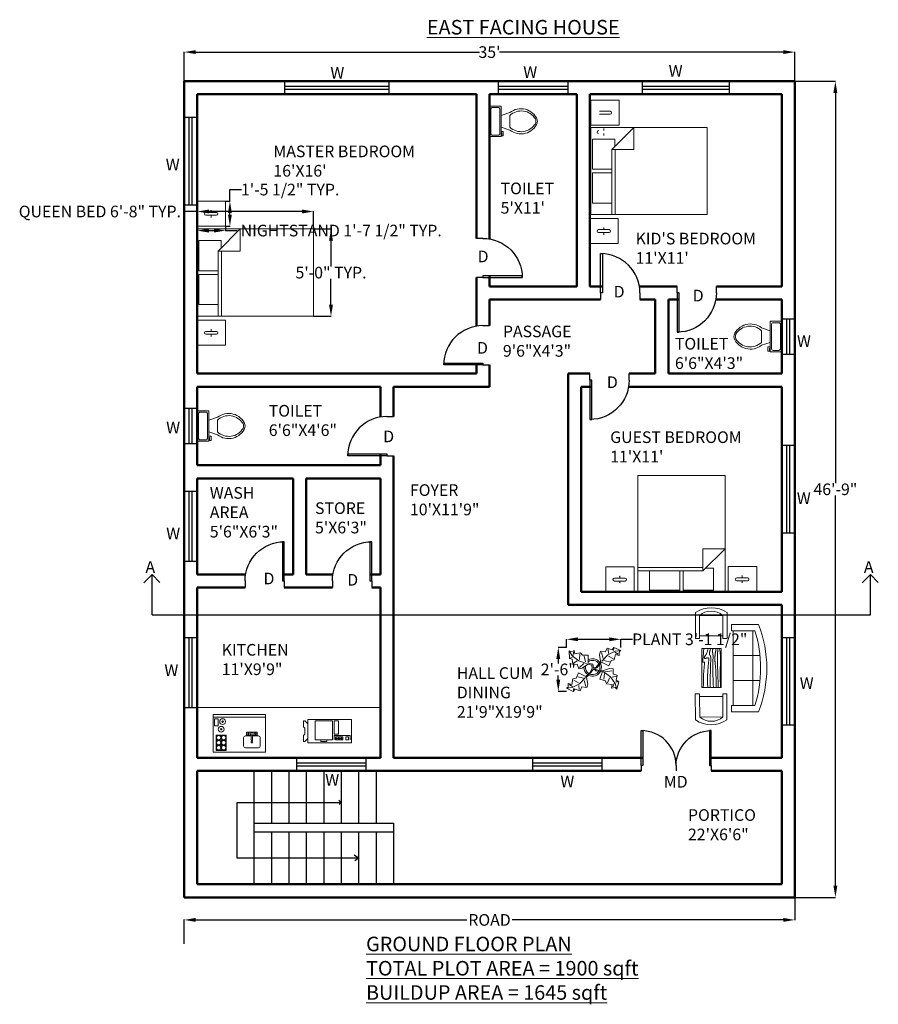
# Model space of a CAD drawing. Units: inches. Extents: x 179 to 2009, y 628 to 2084.
# Tile 1 of 5: x 179 to 769, y 628 to 1305. Entities that reach past the tile are written whole.
import ezdxf

# ---------------------------------------------------------------- set-up
doc = ezdxf.new("R2010")
doc.units = ezdxf.units.IN
doc.header["$MEASUREMENT"] = 0
for name, color, linetype, lineweight in [('A-ANNO-DIMS', 2, 'Continuous', 18), ('A-ANNO-SYMB', 5, 'Continuous', 25), ('A-ANNO-TEXT', 7, 'Continuous', 18), ('A-DOOR', 3, 'Continuous', 25), ('A-FLOR-STRS', 6, 'Continuous', 25), ('A-FURN', 4, 'Continuous', 18), ('A-GLAZ', 2, 'Continuous', 25), ('A-WALL', 1, 'Continuous', 50)]:
    doc.layers.add(name, color=color, linetype=linetype, lineweight=lineweight)
doc.styles.get("Standard").update_dxf_attribs({"font": 'arial.ttf'})
doc.dimstyles.get("Standard").update_dxf_attribs({"dimtxt": 8, "dimasz": 8, "dimexe": 0.18, "dimexo": 0.0625, "dimgap": 0.09, "dimtad": 0, "dimtih": 1, "dimtoh": 1, "dimdec": 0, "dimzin": 0, "dimdsep": 46, "dimlunit": 3, "dimtxsty": 'Standard', "dimcen": 0.09, "dimadec": 0, "dimazin": 0, "dimtfac": 1, "dimtdec": 0, "dimtofl": 0, "dimtmove": 0, "dimatfit": 3, "dimfxl": 1, "dimtolj": 1, "dimtzin": 0, "dimarcsym": 0})

# ---------------------------------------------------------------- blocks, each defined once
blk = doc.blocks.new('*U4')
for p, q in [((0, 0), (0, -6)), ((36, 0), (36, -6))]:
    blk.add_line(p, q)
blk.add_lwpolyline([(0, 0), (0, 36), (1.75, 36), (1.75, 0)], close=True)
blk.add_arc((0, 0), 36, 0, 90)
blk = doc.blocks.new('*U1')
for p, q in [((0, 0), (0, -6)), ((40, 0), (40, -6))]:
    blk.add_line(p, q)
blk.add_lwpolyline([(0, 0), (0, 40), (1.75, 40), (1.75, 0)], close=True)
blk.add_arc((0, 0), 40, 0, 90)
blk = doc.blocks.new('Bed - Queen')
for p, q in [((0, -80.00003), (0, 0)), ((0, 0), (59.99999, 0)), ((59.99999, 0), (59.99999, -80.00003)), ((7.99999, -1.2), (28.79998, -1.2)), ((7.99999, -14.4), (7.99999, -1.2)), ((28.79998, -1.2), (28.79998, -14.4)), ((31.19999, -1.2), (51.99999, -1.2)), ((31.19999, -14.4), (31.19999, -1.2)), ((51.99999, -1.2), (51.99999, -16.4)), ((0, -14.4), (44.8, -14.4)), ((44.8, -16.8), (0, -16.8)), ((59.99999, -29.6), (44.8, -14.4)), ((44.8, -14.4), (44.8, -29.6)), ((51.99999, -16.4), (46.79936, -16.4)), ((44.8, -29.6), (59.99999, -29.6)), ((59.99999, -80.00003), (0, -80.00003))]:
    blk.add_line(p, q)
blk = doc.blocks.new('*U3')
for p, q in [((9.5, -6), (9.5, -2)), ((-10, -8.5), (-8, -8.5)), ((-10, -9.5), (-10, -8.5)), ((-7, -9.5), (-10, -9.5)), ((-8, -8.5), (-8, -8)), ((-7, -8), (-7, -9.5)), ((-4, -8), (-6, -14)), ((4, -8), (6, -14)), ((4, -14), (-4, -14))]:
    blk.add_line(p, q)
blk.add_lwpolyline([(10.5, -8), (10.5, 0), (-10.5, 0), (-10.5, -8)], close=True)
for points in [[(-9.5, -2), (-9.5, -6)], [(8.5, -1), (-8.5, -1)], [(-8.5, -7), (8.5, -7)]]:
    blk.add_lwpolyline(points)
for centre, radius, start, end in [((-8.62, -1.88), 0.884, 81.8699, 188.1301), ((-8.62, -6.12), 0.884, 171.8699, 278.1301), ((8.62, -1.88), 0.884, 351.8699, 98.1301), ((8.62, -6.12), 0.884, 261.8699, 8.1301), ((3.52, -21.58), 12.17, 141.46911, 247.97143), ((4.2, -21.82), 11.33, 136.36773, 238.94682), ((-3.52, -21.58), 12.17, 292.02843, 38.53071), ((-4.2, -21.82), 11.33, 301.05301, 43.63209), ((0, -27.88), 4, 245.73182, 294.26817), ((0, -29), 4, 254.86053, 285.13947)]:
    blk.add_arc(centre, radius, start, end)
blk = doc.blocks.new('Wet Bar')
for p, q in [((0, 0), (36, 0)), ((0, -26), (0, 0)), ((36, 0), (36, -26)), ((0, -2), (36, -2)), ((3.5, -3), (1, -3)), ((1, -3), (1, -8)), ((3.5, -8), (3.5, -3)), ((1, -8), (3.5, -8)), ((2, -14.25), (9, -14.25)), ((2, -24.75), (2, -14.25)), ((2, -17.75), (9, -17.75)), ((5.5, -14.25), (5.5, -24.75)), ((9, -14.25), (9, -24.75)), ((26.2, -17.55), (26.2, -14.1284)), ((27.1001, -17.55), (27.1001, -14.1284)), ((36, -26), (0, -26)), ((9, -21.25), (2, -21.25)), ((9, -24.75), (2, -24.75))]:
    blk.add_line(p, q)
for points in [[(26.2, -14.25), (22.95, -14.25), (22.95, -12.2), (26.75, -12.2)], [(26.7487, -12.2), (30.3501, -12.2), (30.3501, -14.25), (27.1001, -14.25)], [(20.95, -21.75), (20.95, -16.05)], [(22.15, -14.85), (26.2, -14.85)], [(27.1001, -14.85), (31.15, -14.85)], [(32.3501, -16.05), (32.3501, -21.75)], [(31.15, -22.95), (22.15, -22.95)]]:
    blk.add_lwpolyline(points)
for centre, radius in [((6.5, -5), 2), ((6.5, -5), 0.5), ((5.5, -10.25), 2), ((5.5, -10.25), 0.5), ((24.25, -13.25), 0.5), ((26.65, -13.35), 0.9), ((29, -13.25), 0.5), ((3.75, -16), 1.5), ((3.75, -19.5), 1.5), ((7.25, -16), 1.5), ((7.25, -19.5), 1.5), ((26.65, -19.05), 0.6), ((3.75, -23), 1.5), ((7.25, -23), 1.5)]:
    blk.add_circle(centre, radius)
for centre, radius, start, end in [((22.2251, -16.125), 1.2772, 93.36646, 176.6335), ((26.65, -17.55), 0.45, 180, 0), ((31.075, -16.125), 1.2772, 3.366461, 86.63354), ((22.2251, -21.675), 1.2772, 183.3665, 266.6335), ((31.075, -21.675), 1.2772, 273.3665, 356.6335)]:
    blk.add_arc(centre, radius, start, end)
blk = doc.blocks.new('Copy Machine')
for p, q in [((0, 0), (0, -16)), ((30, 0), (0, 0)), ((30, -16), (30, 0)), ((-3, -1), (-3, -5)), ((-2, -1), (-3, -1)), ((-3, -5), (-2, -6)), ((0, -3), (-2, -1)), ((-2, -10), (-2, -6)), ((5, -1), (5, -14)), ((17, -1), (5, -1)), ((17, -14), (17, -1)), ((18, -1), (18, -10)), ((21, -1), (18, -1)), ((21, -10), (21, -1)), ((-3, -11), (-2, -10)), ((-3, -15), (-3, -11)), ((0, -13), (-2, -15)), ((18, -10), (21, -10)), ((18, -14), (18, -11)), ((18, -11), (29, -11)), ((24, -12), (19, -12)), ((19, -12), (19, -14)), ((24, -13), (19, -13)), ((20, -12), (20, -14)), ((21, -14), (21, -12)), ((22, -12), (22, -14)), ((23, -14), (23, -12)), ((24, -14), (24, -12)), ((28, -12), (26, -12)), ((26, -12), (26, -14)), ((28, -14), (28, -12)), ((29, -11), (29, -14)), ((-2, -15), (-3, -15)), ((0, -16), (30, -16)), ((5, -14), (17, -14)), ((9, -14), (9, -15)), ((9, -15), (13, -15)), ((13, -15), (13, -14)), ((19, -14), (24, -14)), ((26, -14), (28, -14))]:
    blk.add_line(p, q)
blk = doc.blocks.new('Sofa - Roundback 7 ft.')
for p, q in [((-12.00002, -32.4421), (-12.00003, -6.5971)), ((11.99997, -32.4421), (11.99998, -6.5971)), ((-36.000027, -34), (-36.000027, -11.4696)), ((-35.999844, -13.3819), (35.9998, -13.3819)), ((35.99998, -34), (35.99998, -11.4696)), ((-36.000027, -32.4421), (35.99998, -32.4421))]:
    blk.add_line(p, q)
for points in [[(-36.000027, -34), (-42.000027, -34), (-42.000027, -8)], [(41.99998, -8), (41.99998, -34), (35.99998, -34)]]:
    blk.add_lwpolyline(points)
for centre, radius, start, end in [((0, -114.25), 114.25, 68.43141, 111.5686), ((-0.00001, -127.1968), 121.1968, 72.72033, 107.2797)]:
    blk.add_arc(centre, radius, start, end)
blk = doc.blocks.new('Table - Rectangular Woodgrain 60 x 30 in.')
for p, q in [((0, 0), (0, -30)), ((60, 0), (0, 0)), ((60, -30), (60, 0)), ((0, -30), (60, -30))]:
    blk.add_line(p, q)
for points in [[(0, -2.4), (4.8155, -2.418), (9.0302, -2.4688), (12.709, -2.5477), (15.9167, -2.65), (18.7181, -2.7711), (21.1781, -2.9063), (23.3616, -3.0508), (25.3333, -3.2), (27.1477, -3.3495), (28.8172, -3.4958), (30.3437, -3.636), (31.7291, -3.7667), (32.9756, -3.8849), (34.0849, -3.9875), (35.059, -4.0714), (35.9, -4.1334), (36.6114, -4.1711), (37.2041, -4.1854), (37.6906, -4.1779), (38.0833, -4.15), (38.3948, -4.1034), (38.6375, -4.0396), (38.8239, -3.9602), (38.9666, -3.8667), (39.0764, -3.7608), (39.1573, -3.6448), (39.2116, -3.521), (39.2416, -3.3917), (39.2498, -3.2593), (39.2385, -3.1261), (39.21, -2.9944), (39.1666, -2.8667), (39.111, -2.7447), (39.0468, -2.6281), (38.978, -2.5163), (38.9083, -2.4083), (38.8418, -2.3035), (38.7823, -2.201), (38.7337, -2.1001), (38.7, -2), (38.6844, -1.9003), (38.6875, -1.8021), (38.7094, -1.707), (38.75, -1.6167), (38.8094, -1.5326), (38.8875, -1.4563), (38.9844, -1.3893), (39.1, -1.3333), (39.2351, -1.2896), (39.3937, -1.2583), (39.5804, -1.2396), (39.8, -1.2333), (40.057, -1.2396), (40.3562, -1.2583), (40.7023, -1.2896), (41.1, -1.3333), (41.5547, -1.3895), (42.0755, -1.4573), (42.6721, -1.5361), (43.3542, -1.625), (44.1316, -1.7233), (45.014, -1.8302), (46.0114, -1.9449), (47.1333, -2.0667), (48.3862, -2.1947), (49.7625, -2.3281), (51.2513, -2.4663), (52.8416, -2.6083), (54.5226, -2.7535), (56.2833, -2.9011), (58.1127, -3.0501), (60, -3.2)], [(0, -9.2), (6.5759, -9.0858), (11.9385, -9.0365), (16.2527, -9.0418), (19.6833, -9.0917), (22.3952, -9.1759), (24.5531, -9.2844), (26.322, -9.4069), (27.8666, -9.5333), (29.3241, -9.6553), (30.7203, -9.7719), (32.0532, -9.8837), (33.3208, -9.9917), (34.5213, -10.0965), (35.6526, -10.199), (36.7128, -10.2999), (37.7, -10.4), (38.6129, -10.4996), (39.4531, -10.5969), (40.223, -10.6895), (40.925, -10.775), (41.5613, -10.8512), (42.1344, -10.9156), (42.6465, -10.966), (43.1, -11), (43.4976, -11.0158), (43.8437, -11.0136), (44.143, -10.9942), (44.4, -10.9583), (44.6195, -10.9069), (44.8062, -10.8406), (44.9648, -10.7603), (45.1, -10.6667), (45.2155, -10.5598), (45.3114, -10.4365), (45.3871, -10.2929), (45.4416, -10.125), (45.4743, -9.929), (45.4844, -9.7011), (45.4709, -9.4371), (45.4333, -9.1333), (45.3716, -8.7883), (45.2896, -8.4104), (45.1919, -8.0107), (45.0833, -7.6), (44.9685, -7.1893), (44.8521, -6.7896), (44.7388, -6.4117), (44.6333, -6.0667), (44.54, -5.7628), (44.4614, -5.4979), (44.4001, -5.2675), (44.3583, -5.0667), (44.3384, -4.8909), (44.3427, -4.7354), (44.3736, -4.5956), (44.4333, -4.4667), (44.5236, -4.3453), (44.6427, -4.2333), (44.7884, -4.1339), (44.9583, -4.05), (45.1501, -3.9849), (45.3614, -3.9417), (45.59, -3.9234), (45.8333, -3.9333), (46.0915, -3.9749), (46.3734, -4.0531), (46.6906, -4.1736), (47.0542, -4.3417), (47.4756, -4.5629), (47.9661, -4.8427), (48.5372, -5.1866), (49.2, -5.6), (49.9676, -6.0844), (50.8594, -6.625), (51.8965, -7.2031), (53.1, -7.8), (54.491, -8.3969), (56.0906, -8.975), (57.9199, -9.5156), (60, -10)], [(0, -12.8), (5.1847, -12.9322), (9.6213, -13.0323), (13.3963, -13.1059), (16.5958, -13.1583), (19.3063, -13.1952), (21.614, -13.2219), (23.6054, -13.2439), (25.3666, -13.2667), (26.9728, -13.2947), (28.4531, -13.3281), (29.8256, -13.3663), (31.1083, -13.4083), (32.3191, -13.4535), (33.476, -13.501), (34.597, -13.5501), (35.7, -13.6), (36.7984, -13.6497), (37.8875, -13.6979), (38.9578, -13.743), (40, -13.7833), (41.0047, -13.8174), (41.9625, -13.8438), (42.864, -13.8607), (43.7, -13.8667), (44.4631, -13.8604), (45.1552, -13.8417), (45.7801, -13.8104), (46.3416, -13.7667), (46.8439, -13.7104), (47.2906, -13.6417), (47.6858, -13.5604), (48.0333, -13.4667), (48.3375, -13.3608), (48.6042, -13.2448), (48.8396, -13.121), (49.05, -12.9917), (49.2417, -12.8593), (49.4208, -12.7261), (49.5937, -12.5944), (49.7667, -12.4667), (49.9452, -12.3451), (50.1323, -12.2313), (50.3303, -12.1268), (50.5416, -12.0333), (50.7686, -11.9524), (51.0135, -11.8854), (51.2788, -11.8341), (51.5666, -11.8), (51.8785, -11.7843), (52.2116, -11.7865), (52.562, -11.8059), (52.926, -11.8417), (53.2998, -11.8931), (53.6795, -11.9594), (54.0614, -12.0397), (54.4416, -12.1333), (54.8223, -12.2401), (55.2293, -12.3625), (55.6942, -12.5037), (56.2489, -12.6667), (56.9251, -12.8547), (57.7545, -13.0708), (58.7689, -13.3182), (60, -13.6)], [(0, -18), (5.124, -17.7273), (9.6609, -17.5057), (13.6705, -17.3303), (17.2125, -17.1958), (20.3467, -17.0973), (23.1328, -17.0297), (25.6307, -16.9878), (27.9, -16.9667), (29.9928, -16.9617), (31.9302, -16.9703), (33.7254, -16.9907), (35.3917, -17.0208), (36.9423, -17.0588), (38.3906, -17.1026), (39.7499, -17.1503), (41.0333, -17.2), (42.2519, -17.2496), (43.4073, -17.2969), (44.4986, -17.3395), (45.525, -17.375), (46.4858, -17.4012), (47.3802, -17.4156), (48.2074, -17.416), (48.9667, -17.4), (49.6583, -17.3662), (50.2872, -17.3167), (50.8595, -17.2547), (51.3812, -17.1833), (51.8584, -17.1057), (52.2971, -17.025), (52.7034, -16.9443), (53.0833, -16.8667), (53.443, -16.7951), (53.789, -16.7313), (54.128, -16.6768), (54.4666, -16.6334), (54.8115, -16.6024), (55.1693, -16.5854), (55.5465, -16.5841), (55.95, -16.6), (56.3828, -16.6337), (56.8346, -16.6823), (57.2915, -16.7418), (57.7396, -16.8084), (58.165, -16.878), (58.5539, -16.9469), (58.8924, -17.0111), (59.1666, -17.0667), (59.3679, -17.1107), (59.5078, -17.1438), (59.6032, -17.1675), (59.6708, -17.1833), (59.7275, -17.193), (59.7901, -17.1979), (59.8753, -17.1998), (60, -17.2)], [(0, -22.4), (8.0098, -22.2501), (14.4094, -22.1011), (19.4168, -21.9535), (23.25, -21.8083), (26.1269, -21.6663), (28.2656, -21.5281), (29.884, -21.3947), (31.2, -21.2667), (32.3967, -21.1448), (33.5172, -21.0292), (34.5697, -20.9198), (35.5625, -20.8167), (36.5037, -20.7198), (37.4015, -20.6292), (38.2642, -20.5448), (39.1, -20.4667), (39.9164, -20.3951), (40.7187, -20.3313), (41.5117, -20.2768), (42.3, -20.2333), (43.0883, -20.2024), (43.8812, -20.1854), (44.6836, -20.1841), (45.5, -20.2), (46.3328, -20.234), (47.1747, -20.2844), (48.0163, -20.3488), (48.8479, -20.425), (49.66, -20.5106), (50.4429, -20.6031), (51.1872, -20.7004), (51.8833, -20.8), (52.5246, -20.8999), (53.1166, -20.9995), (53.6681, -21.0983), (54.1875, -21.1958), (54.6834, -21.2919), (55.1646, -21.3859), (55.6394, -21.4777), (56.1167, -21.5667), (56.6028, -21.6515), (57.0961, -21.7266), (57.5929, -21.7852), (58.0896, -21.8208), (58.5823, -21.8268), (59.0674, -21.7964), (59.5412, -21.723), (60, -21.6)], [(0, -25.2), (8.6355, -25.0504), (15.7026, -24.9031), (21.4049, -24.7606), (25.9458, -24.625), (29.529, -24.4988), (32.3578, -24.3844), (34.6359, -24.284), (36.5667, -24.2), (38.3213, -24.1341), (39.9417, -24.0854), (41.437, -24.0523), (42.8167, -24.0333), (44.0901, -24.0268), (45.2667, -24.0313), (46.3557, -24.0451), (47.3667, -24.0667), (48.309, -24.0947), (49.1928, -24.1287), (50.0284, -24.168), (50.826, -24.2125), (51.5959, -24.2617), (52.3483, -24.3151), (53.0935, -24.3725), (53.8417, -24.4334), (54.6009, -24.497), (55.3699, -24.561), (56.1454, -24.6226), (56.9239, -24.6792), (57.7021, -24.7279), (58.4764, -24.7662), (59.2435, -24.7911), (60, -24.8)], [(0, -28.8), (5.6867, -28.6681), (10.45, -28.5698), (14.407, -28.5012), (17.675, -28.4584), (20.3711, -28.4374), (22.6125, -28.4344), (24.5164, -28.4455), (26.2, -28.4667), (27.762, -28.4947), (29.2276, -28.5281), (30.6033, -28.5663), (31.8958, -28.6084), (33.1118, -28.6535), (34.2578, -28.7011), (35.3405, -28.7501), (36.3666, -28.8), (37.3443, -28.8497), (38.288, -28.8974), (39.2137, -28.9412), (40.1375, -28.9792), (41.0753, -29.0093), (42.0432, -29.0297), (43.0572, -29.0384), (44.1333, -29.0333), (45.2936, -29.0114), (46.5843, -28.9641), (48.0579, -28.8816), (49.7666, -28.7542), (51.7629, -28.5721), (54.0989, -28.3255), (56.8272, -28.0048), (60, -27.6)]]:
    blk.add_lwpolyline(points)
blk = doc.blocks.new('Plant - Rubber or Philodendron')
for p, q in [((13.3837, 12.301), (14.68, 13.9039)), ((14.68, 13.9039), (19.3848, 11.8146)), ((-16.2005, 11.4774), (-13.9899, 8.1064)), ((-16.2005, 11.4774), (-14.8639, 10.7964)), ((-16.0159, 6.3329), (-16.2005, 11.4774)), ((-15.3434, 6.5514), (-13.9984, 6.9884)), ((-14.8639, 10.7964), (-12.6195, 11.8975)), ((-13.9899, 8.1064), (-9.5434, 4.7185)), ((-13.3174, 8.325), (-13.0735, 11.0065)), ((-12.6195, 11.8975), (-12.1909, 9.4345)), ((-12.1909, 9.4345), (-8.3829, 10.3)), ((-8.8369, 9.409), (-9.0894, 5.6095)), ((-8.3829, 10.3), (-7.0549, 8.501)), ((-7.0549, 8.501), (-3.0284, 8.6941)), ((-4.8529, 4.012), (-5.7184, 7.82)), ((-3.0284, 8.6941), (-3.0709, 3.1041)), ((4.6914, 8.8812), (5.3859, 11.2828)), ((4.6914, 8.8812), (5.5014, 4.4831)), ((5.3859, 11.2828), (8.8871, 10.7908)), ((5.9878, 10.4842), (7.1971, 6.3869)), ((10.3916, 8.7942), (6.2847, 4.4028)), ((8.8871, 10.7908), (9.9809, 13.4933)), ((9.9809, 13.4933), (13.3837, 12.301)), ((15.3859, 11.3055), (10.3916, 8.7942)), ((10.5828, 12.6946), (10.8893, 9.7953)), ((14.2977, 6.1031), (10.9934, 7.9956)), ((14.5816, 13.2037), (14.3848, 11.8033)), ((15.7909, 9.1065), (14.8995, 5.3044)), ((15.2875, 10.6053), (17.5907, 9.2105)), ((19.3848, 11.8146), (15.3859, 11.3055)), ((18.1925, 8.4119), (15.7909, 9.1065)), ((19.3848, 11.8146), (18.1868, 10.9119)), ((18.1868, 10.9119), (18.1925, 8.4119)), ((-14.0069, 5.8704), (-16.0159, 6.3329)), ((-13.5868, 2.2894), (-14.0069, 5.8704)), ((-10.6784, 2.491), (-13.5868, 2.2894)), ((-13.1329, 3.1804), (-10.6614, 4.727)), ((-9.5858, -0.8715), (-10.6784, 2.491)), ((-9.5434, 4.7185), (-4.1917, 2.9888)), ((-9.1318, 0.0195), (-5.9793, 2.9025)), ((-7.1228, -0.443), (-3.5248, 2.2131)), ((-3.5248, 2.2131), (-3.3011, 2.4355)), ((-3.3011, 2.4355), (-0.5306, 1.7947)), ((-3.0709, 3.1041), (0.0797, 2.3163)), ((-0.5306, 1.7947), (-0.2255, -0.5527)), ((-0.5306, 1.7947), (-0.5306, 1.7947)), ((0.0797, 2.3163), (0.4866, -0.031)), ((0.4866, -0.031), (2.1141, 0.2298)), ((2.1141, 0.2298), (5.4346, 3.9146)), ((6.1032, 3.6844), (2.8262, -0.031)), ((5.4346, 3.9146), (5.5014, 4.4831)), ((11.1089, 1.1958), (6.1032, 3.6844)), ((7.7005, 4.8881), (11.5025, 3.9967)), ((12.7005, 4.8994), (11.1089, 1.1958)), ((14.8995, 5.3044), (12.7005, 4.8994)), ((-11.3237, -7.2629), (-9.7321, -3.5593)), ((-6.3237, -7.2516), (-10.1257, -6.3602)), ((-9.7321, -3.5593), (-4.7264, -6.0479)), ((-7.1228, -0.443), (-9.5858, -0.8715)), ((-2.019, -3.6148), (-4.7264, -6.0479)), ((-4.1246, -6.8466), (-4.0579, -6.2781)), ((-4.0579, -6.2781), (-0.9375, -3.1608)), ((-2.019, -3.6148), (-0.2255, -0.5527)), ((-0.9375, -3.1608), (0.5883, -0.8135)), ((0.5883, -0.8135), (2.2447, -2.0916)), ((2.8262, -0.031), (1.3003, -0.5527)), ((1.3003, -0.5527), (2.4193, -1.4655)), ((2.2447, -2.0916), (6.7108, -2.6626)), ((2.4193, -1.4655), (6.895, -2.1175)), ((4.943, -7.9659), (6.7108, -2.6626)), ((11.6605, -0.5413), (6.895, -2.1175)), ((12.3677, -6.1981), (7.219, -2.6772)), ((8.125, -4.0768), (7.7715, -7.9659)), ((8.3544, -2.7453), (13.1973, -2.1704)), ((11.6605, -0.5413), (14.1354, -0.8948)), ((15.5496, -10.7943), (12.3677, -6.1981)), ((16.2567, -5.8446), (13.4283, -6.5517)), ((14.1354, -0.8948), (14.1354, -4.4304)), ((14.1354, -4.4304), (16.9638, -5.1375)), ((16.9638, -5.1375), (16.2567, -8.673)), ((-18.008, -14.1781), (-16.8101, -13.2754)), ((-16.8157, -10.7754), (-14.4141, -11.4699)), ((-16.8101, -13.2754), (-16.8157, -10.7754)), ((-13.9107, -12.9688), (-16.2139, -11.574)), ((-14.4141, -11.4699), (-13.5228, -7.6679)), ((-14.0091, -13.669), (-9.0148, -11.1577)), ((-13.5228, -7.6679), (-11.3237, -7.2629)), ((-12.921, -8.4665), (-9.6166, -10.359)), ((-9.206, -15.0581), (-9.5126, -12.1588)), ((-9.0148, -11.1577), (-4.9047, -6.8122)), ((-7.5103, -13.1543), (-8.6042, -15.8568)), ((-4.0092, -13.6463), (-7.5103, -13.1543)), ((-4.611, -12.8477), (-5.8203, -8.7504)), ((-3.3146, -11.2447), (-4.1246, -6.8466)), ((-3.3146, -11.2447), (-4.0092, -13.6463)), ((8.8321, -9.0266), (4.943, -7.9659)), ((9.5392, -11.1479), (8.8321, -9.0266)), ((13.4283, -11.5015), (9.5392, -11.1479)), ((10.2463, -10.4408), (11.6605, -6.9053)), ((13.0748, -13.9763), (13.4283, -11.5015)), ((14.8425, -10.7943), (13.7819, -13.2692)), ((16.6103, -14.6834), (15.5496, -10.7943)), ((17.3174, -9.7337), (15.9032, -9.7337)), ((16.2567, -8.673), (18.0245, -9.7337)), ((18.0245, -9.7337), (16.6103, -14.6834)), ((-18.008, -14.1781), (-14.0091, -13.669)), ((-13.3032, -16.2674), (-18.008, -14.1781)), ((-12.0069, -14.6645), (-13.3032, -16.2674)), ((-13.2048, -15.5672), (-13.008, -14.1668)), ((-8.6042, -15.8568), (-12.0069, -14.6645)), ((15.5496, -13.6228), (13.0748, -13.9763)), ((16.6103, -14.6834), (15.5496, -13.6228))]:
    blk.add_line(p, q)
for centre, radius, start, end in [((0.0308, 0.1664), 6, 178.6147, 235.1169), ((0.0308, 0.1664), 5, 168.1647, 238.6725), ((0, 0), 6.1275, 34.37569, 120.1028), ((-0.0601, -0.2075), 5.2461, 33.82192, 124.9414), ((-0.2664, 0.1682), 5.2775, 338.4094, 20.03007), ((-0.098, 0.1364), 6.1288, 341.2017, 26.09184), ((-0.0234, 0.3825), 6.1492, 242.5812, 331.2714), ((-0.1102, 0.4886), 5.2883, 247.3711, 327.472)]:
    blk.add_arc(centre, radius, start, end)
blk = doc.blocks.new('*D14')
at = {"layer": 'A-ANNO-DIMS', "color": 0, "lineweight": -2, "transparency": 16777216}
for p, q in [((291.69, 1262.41), (291.69, 1282.56)), ((299.69, 1282.38), (494.81, 1282.38)), ((703.69, 1282.38), (508.56, 1282.38)), ((711.69, 1262.41), (711.69, 1282.56))]:
    blk.add_line(p, q, dxfattribs=at)
at = {"layer": 'A-ANNO-DIMS', "color": 0, "transparency": 16777216}
for points in [[(299.69, 1283.72), (299.69, 1281.05), (291.69, 1282.38)], [(703.69, 1283.72), (703.69, 1281.05), (711.69, 1282.38)]]:
    blk.add_solid(points, dxfattribs=at)
at = {"layer": 'Defpoints', "color": 0, "transparency": 16777216}
for p in [(711.69, 1282.38), (291.69, 1262.35), (711.69, 1262.35)]:
    blk.add_point(p, dxfattribs=at)
at = {"layer": 'A-ANNO-DIMS', "color": 0, "transparency": 16777216, "insert": (501.69, 1282.38), "char_height": 8, "attachment_point": 5}
blk.add_mtext("\\A1;35'", dxfattribs=at)
blk = doc.blocks.new('*D15')
at = {"layer": 'A-ANNO-DIMS', "color": 0, "lineweight": -2, "transparency": 16777216}
for p, q in [((711.75, 1262.35), (739.72, 1262.35)), ((739.54, 1254.35), (739.54, 986.02)), ((739.54, 709.35), (739.54, 977.68)), ((711.75, 701.35), (739.72, 701.35))]:
    blk.add_line(p, q, dxfattribs=at)
at = {"layer": 'A-ANNO-DIMS', "color": 0, "transparency": 16777216}
for points in [[(738.2, 1254.35), (740.87, 1254.35), (739.54, 1262.35)], [(738.2, 709.35), (740.87, 709.35), (739.54, 701.35)]]:
    blk.add_solid(points, dxfattribs=at)
at = {"layer": 'Defpoints', "color": 0, "transparency": 16777216}
for p in [(711.69, 1262.35), (711.69, 701.35), (739.54, 701.35)]:
    blk.add_point(p, dxfattribs=at)
at = {"layer": 'A-ANNO-DIMS', "color": 0, "transparency": 16777216, "insert": (739.54, 981.85), "char_height": 8, "attachment_point": 5}
blk.add_mtext('\\A1;46\'-9"', dxfattribs=at)
blk = doc.blocks.new('*D16')
at = {"layer": 'A-ANNO-DIMS', "color": 0, "lineweight": -2, "transparency": 16777216}
for p, q in [((711.69, 701.29), (711.69, 685.68)), ((291.69, 669.31), (291.69, 686.04)), ((299.69, 685.86), (486.19, 685.86)), ((703.69, 685.86), (517.18, 685.86))]:
    blk.add_line(p, q, dxfattribs=at)
at = {"layer": 'A-ANNO-DIMS', "color": 0, "transparency": 16777216}
for points in [[(299.69, 687.2), (299.69, 684.53), (291.69, 685.86)], [(703.69, 687.2), (703.69, 684.53), (711.69, 685.86)]]:
    blk.add_solid(points, dxfattribs=at)
at = {"layer": 'Defpoints', "color": 0, "transparency": 16777216}
for p in [(711.69, 701.35), (711.69, 685.86), (291.69, 669.25)]:
    blk.add_point(p, dxfattribs=at)
at = {"layer": 'A-ANNO-DIMS', "color": 0, "transparency": 16777216, "insert": (501.69, 685.86), "char_height": 8, "attachment_point": 5}
blk.add_mtext('\\A1;ROAD', dxfattribs=at)
blk = doc.blocks.new('ARMCHAIR')
for p, q in [((0, 0), (0, 17.87)), ((2.68, 1.83), (2.68, 15.94)), ((2.68, 15.94), (18.72, 15.94)), ((18.72, 15.94), (18.72, 1.83)), ((21.68, 0), (21.68, 17.87)), ((2.68, 0), (0, 0)), ((18.72, 1.83), (2.68, 1.83)), ((2.68, 1.83), (2.68, 0)), ((18.72, 1.83), (18.72, 0)), ((18.72, 0), (21.68, 0))]:
    blk.add_line(p, q)
for centre, radius, start, end in [((10.84, 2.23), 19.03, 55.27776, 124.72224), ((10.7, 6.48), 12.4, 49.71958, 130.28042)]:
    blk.add_arc(centre, radius, start, end)
blk = doc.blocks.new('NIGHTSTAND-2')
for p, q in [((5.95, 9.55), (13.25, 9.55)), ((5.95, 7.55), (13.25, 7.55)), ((9.6, 10.86), (9.43, 10.74)), ((9.6, 9.55), (9.6, 10.86)), ((9.6, 10.86), (9.78, 10.74)), ((9.6, 7.55), (9.6, 6.33)), ((9.6, 6.33), (9.37, 6.5)), ((9.6, 6.33), (9.83, 6.48))]:
    blk.add_line(p, q)
blk.add_lwpolyline([(0, 17.25), (19.57, 17.25), (19.57, 0), (0, 0)], close=True)
for centre, start, end in [((5.95, 8.55), 90, 270), ((13.25, 8.55), 270, 90)]:
    blk.add_arc(centre, 1, start, end)
blk = doc.blocks.new('*D43')
at = {"layer": 'A-ANNO-DIMS', "color": 0, "lineweight": -2, "transparency": 16777216}
for p, q in [((300.69, 1172.8), (292.69, 1172.8)), ((300.69, 1160.87), (300.69, 1172.98)), ((372.69, 1172.8), (308.69, 1172.8)), ((380.69, 1160.87), (380.69, 1172.98))]:
    blk.add_line(p, q, dxfattribs=at)
at = {"layer": 'A-ANNO-DIMS', "color": 0, "transparency": 16777216}
for points in [[(308.69, 1174.14), (308.69, 1171.47), (300.69, 1172.8)], [(372.69, 1174.14), (372.69, 1171.47), (380.69, 1172.8)]]:
    blk.add_solid(points, dxfattribs=at)
at = {"layer": 'Defpoints', "color": 0, "transparency": 16777216}
for p in [(300.69, 1172.8), (300.69, 1160.8), (380.69, 1160.8)]:
    blk.add_point(p, dxfattribs=at)
at = {"layer": 'A-ANNO-DIMS', "color": 0, "transparency": 16777216, "insert": (233.76, 1172.8), "char_height": 8, "attachment_point": 5}
blk.add_mtext('\\A1;QUEEN BED 6\'-8" TYP.', dxfattribs=at)
blk = doc.blocks.new('*D44')
at = {"layer": 'A-ANNO-DIMS', "color": 0, "lineweight": -2, "transparency": 16777216}
for p, q in [((380.75, 1160.8), (392.87, 1160.8)), ((392.69, 1152.8), (392.69, 1134.98)), ((392.69, 1108.8), (392.69, 1126.63)), ((380.75, 1100.8), (392.87, 1100.8))]:
    blk.add_line(p, q, dxfattribs=at)
at = {"layer": 'A-ANNO-DIMS', "color": 0, "transparency": 16777216}
for points in [[(391.35, 1152.8), (394.02, 1152.8), (392.69, 1160.8)], [(391.35, 1108.8), (394.02, 1108.8), (392.69, 1100.8)]]:
    blk.add_solid(points, dxfattribs=at)
at = {"layer": 'Defpoints', "color": 0, "transparency": 16777216}
for p in [(380.69, 1160.8), (392.69, 1160.8), (380.69, 1100.8)]:
    blk.add_point(p, dxfattribs=at)
at = {"layer": 'A-ANNO-DIMS', "color": 0, "transparency": 16777216, "insert": (392.69, 1130.8), "char_height": 8, "attachment_point": 5}
blk.add_mtext('\\A1;5\'-0" TYP.', dxfattribs=at)
blk = doc.blocks.new('*D49')
at = {"layer": 'A-ANNO-DIMS', "color": 0, "lineweight": -2, "transparency": 16777216}
for p, q in [((300.69, 1162.57), (300.69, 1159.52)), ((308.69, 1159.7), (312.25, 1159.7)), ((320.25, 1162.57), (320.25, 1159.52)), ((320.25, 1159.7), (328.25, 1159.7))]:
    blk.add_line(p, q, dxfattribs=at)
at = {"layer": 'A-ANNO-DIMS', "color": 0, "transparency": 16777216}
for points in [[(308.69, 1161.03), (308.69, 1158.36), (300.69, 1159.7)], [(312.25, 1161.03), (312.25, 1158.36), (320.25, 1159.7)]]:
    blk.add_solid(points, dxfattribs=at)
at = {"layer": 'Defpoints', "color": 0, "transparency": 16777216}
for p in [(300.69, 1162.63), (320.25, 1162.63), (320.25, 1159.7)]:
    blk.add_point(p, dxfattribs=at)
at = {"layer": 'A-ANNO-DIMS', "color": 0, "transparency": 16777216, "insert": (399.73, 1159.7), "char_height": 8, "attachment_point": 5}
blk.add_mtext('\\A1;NIGHTSTAND 1\'-7 1/2" TYP.', dxfattribs=at)
blk = doc.blocks.new('*D50')
at = {"layer": 'A-ANNO-DIMS', "color": 0, "lineweight": -2, "transparency": 16777216}
for p, q in [((323.19, 1179.88), (323.19, 1187.88)), ((323.19, 1187.88), (331.19, 1187.88)), ((320.31, 1179.88), (323.37, 1179.88)), ((323.19, 1170.63), (323.19, 1171.88)), ((320.31, 1162.63), (323.37, 1162.63))]:
    blk.add_line(p, q, dxfattribs=at)
at = {"layer": 'A-ANNO-DIMS', "color": 0, "transparency": 16777216}
for points in [[(321.85, 1171.88), (324.52, 1171.88), (323.19, 1179.88)], [(321.85, 1170.63), (324.52, 1170.63), (323.19, 1162.63)]]:
    blk.add_solid(points, dxfattribs=at)
at = {"layer": 'Defpoints', "color": 0, "transparency": 16777216}
for p in [(320.25, 1179.88), (323.19, 1179.88), (320.25, 1162.63)]:
    blk.add_point(p, dxfattribs=at)
at = {"layer": 'A-ANNO-DIMS', "color": 0, "transparency": 16777216, "insert": (364.6, 1187.88), "char_height": 8, "attachment_point": 5}
blk.add_mtext('\\A1;1\'-5 1/2" TYP.', dxfattribs=at)
blk = doc.blocks.new('*D61')
at = {"layer": 'A-ANNO-DIMS', "color": 0, "lineweight": -2, "transparency": 16777216}
for p, q in [((554.6, 873.19), (554.6, 878.92)), ((562.6, 878.74), (583.99, 878.74)), ((591.99, 873.19), (591.99, 878.92)), ((591.99, 878.74), (599.99, 878.74))]:
    blk.add_line(p, q, dxfattribs=at)
at = {"layer": 'A-ANNO-DIMS', "color": 0, "transparency": 16777216}
for points in [[(562.6, 880.07), (562.6, 877.41), (554.6, 878.74)], [(583.99, 880.07), (583.99, 877.41), (591.99, 878.74)]]:
    blk.add_solid(points, dxfattribs=at)
at = {"layer": 'Defpoints', "color": 0, "transparency": 16777216}
for p in [(554.6, 873.13), (591.99, 878.74), (591.99, 873.13)]:
    blk.add_point(p, dxfattribs=at)
at = {"layer": 'A-ANNO-DIMS', "color": 0, "transparency": 16777216, "insert": (639.4, 878.74), "char_height": 8, "attachment_point": 5}
blk.add_mtext('\\A1;PLANT 3\'-1 1/2"', dxfattribs=at)
blk = doc.blocks.new('*D62')
at = {"layer": 'A-ANNO-DIMS', "color": 0, "lineweight": -2, "transparency": 16777216}
for p, q in [((554.53, 873.13), (548.81, 873.13)), ((548.99, 865.13), (548.99, 862.22)), ((548.99, 850.96), (548.99, 853.87)), ((554.53, 842.96), (548.81, 842.96))]:
    blk.add_line(p, q, dxfattribs=at)
at = {"layer": 'A-ANNO-DIMS', "color": 0, "transparency": 16777216}
for points in [[(547.65, 865.13), (550.32, 865.13), (548.99, 873.13)], [(547.65, 850.96), (550.32, 850.96), (548.99, 842.96)]]:
    blk.add_solid(points, dxfattribs=at)
at = {"layer": 'Defpoints', "color": 0, "transparency": 16777216}
for p in [(548.99, 873.13), (554.6, 873.13), (554.6, 842.96)]:
    blk.add_point(p, dxfattribs=at)
at = {"layer": 'A-ANNO-DIMS', "color": 0, "transparency": 16777216, "insert": (548.99, 858.04), "char_height": 8, "attachment_point": 5}
blk.add_mtext('\\A1;2\'-6"', dxfattribs=at)

msp = doc.modelspace()

# ---------------------------------------------------------------- linework, layer by layer
at = {"layer": 'A-ANNO-SYMB'}
for p, q in [((269.72, 923.19), (263.96, 917.47)), ((269.72, 895.65), (269.72, 923.19)), ((269.72, 923.19), (275.04, 917.84)), ((763.74, 923.19), (757.98, 917.47)), ((763.74, 895.65), (763.74, 923.19)), ((763.74, 923.19), (769.06, 917.84)), ((269.72, 895.65), (763.74, 895.65))]:
    msp.add_line(p, q, dxfattribs=at)
at = {"layer": 'A-FLOR-STRS'}
for p, q in [((339.69, 788.35), (339.69, 710.35)), ((351.69, 788.35), (351.69, 752.35)), ((363.69, 788.35), (363.69, 752.35)), ((375.69, 788.35), (375.69, 752.35)), ((387.69, 788.35), (387.69, 752.35)), ((399.69, 788.35), (399.69, 752.35)), ((411.69, 788.35), (411.69, 752.35)), ((423.69, 788.35), (423.69, 752.35)), ((328.24, 728.35), (328.24, 766.55)), ((328.24, 766.55), (399.69, 766.55)), ((399.69, 766.55), (398.08, 767.97)), ((399.69, 766.55), (398.32, 765.27)), ((339.69, 752.35), (435.69, 752.35)), ((435.69, 752.35), (435.69, 710.35)), ((339.69, 746.35), (435.69, 746.35)), ((351.69, 746.35), (351.69, 710.35)), ((363.69, 746.35), (363.69, 710.35)), ((375.69, 746.35), (375.69, 710.35)), ((387.69, 746.35), (387.69, 710.35)), ((399.69, 746.35), (399.69, 710.35)), ((411.69, 746.35), (411.69, 710.35)), ((423.69, 746.35), (423.69, 710.35)), ((411.69, 728.35), (328.24, 728.35)), ((411.69, 728.35), (408.72, 730.27)), ((411.69, 728.35), (409.16, 726.46))]:
    msp.add_line(p, q, dxfattribs=at)
at = {"layer": 'A-FURN'}
for p, q in [((577.36, 1241.71), (584.66, 1241.71)), ((577.36, 1239.71), (584.66, 1239.71)), ((580.29, 1225.2), (580.05, 1225.36)), ((580.29, 1229.73), (580.11, 1229.6)), ((580.29, 1228.42), (580.29, 1229.73)), ((580.29, 1229.73), (580.47, 1229.61)), ((580.29, 1226.42), (580.29, 1225.2)), ((580.29, 1225.2), (580.52, 1225.34)), ((300.69, 831.85), (426.69, 831.85))]:
    msp.add_line(p, q, dxfattribs=at)
msp.add_lwpolyline([(571.41, 1249.41), (590.97, 1249.41), (590.97, 1232.16), (571.41, 1232.16)], close=True, dxfattribs=at)
for centre, start, end in [((584.66, 1240.71), 270, 90), ((576.64, 1227.42), 90, 270)]:
    msp.add_arc(centre, 1, start, end, dxfattribs=at)
at = {"layer": 'A-GLAZ'}
for p, q in [((360.69, 1258.85), (432.69, 1258.85)), ((360.69, 1256.85), (432.69, 1256.85)), ((507.69, 1258.85), (555.69, 1258.85)), ((507.69, 1256.85), (555.69, 1256.85)), ((606.69, 1258.85), (666.69, 1258.85)), ((606.69, 1256.85), (666.69, 1256.85)), ((295.19, 1177.46), (295.19, 1237.46)), ((297.19, 1177.46), (297.19, 1237.46)), ((706.19, 1074.85), (706.19, 1098.85)), ((708.19, 1074.85), (708.19, 1098.85)), ((295.19, 1013.35), (295.19, 1037.35)), ((297.19, 1013.35), (297.19, 1037.35)), ((706.19, 951.85), (706.19, 1011.85)), ((708.19, 951.85), (708.19, 1011.85)), ((295.19, 932.35), (295.19, 980.35)), ((297.19, 932.35), (297.19, 980.35)), ((295.19, 831.85), (295.19, 879.85)), ((297.19, 831.85), (297.19, 879.85)), ((706.19, 819.85), (706.19, 879.85)), ((708.19, 819.85), (708.19, 879.85)), ((368.86, 793.85), (416.86, 793.85)), ((531.27, 793.85), (579.27, 793.85)), ((368.86, 791.85), (416.86, 791.85)), ((531.27, 791.85), (579.27, 791.85))]:
    msp.add_line(p, q, dxfattribs=at)
for points in [[(360.69, 1253.35), (432.69, 1253.35), (432.69, 1262.35), (360.69, 1262.35)], [(507.69, 1253.35), (555.69, 1253.35), (555.69, 1262.35), (507.69, 1262.35)], [(606.69, 1253.35), (666.69, 1253.35), (666.69, 1262.35), (606.69, 1262.35)], [(300.69, 1177.46), (300.69, 1237.46), (291.69, 1237.46), (291.69, 1177.46)], [(711.69, 1074.85), (711.69, 1098.85), (702.69, 1098.85), (702.69, 1074.85)], [(300.69, 1013.35), (300.69, 1037.35), (291.69, 1037.35), (291.69, 1013.35)], [(711.69, 951.85), (711.69, 1011.85), (702.69, 1011.85), (702.69, 951.85)], [(300.69, 932.35), (300.69, 980.35), (291.69, 980.35), (291.69, 932.35)], [(300.69, 831.85), (300.69, 879.85), (291.69, 879.85), (291.69, 831.85)], [(711.69, 819.85), (711.69, 879.85), (702.69, 879.85), (702.69, 819.85)], [(368.86, 788.35), (416.86, 788.35), (416.86, 797.35), (368.86, 797.35)], [(531.27, 788.35), (579.27, 788.35), (579.27, 797.35), (531.27, 797.35)]]:
    msp.add_lwpolyline(points, close=True, dxfattribs=at)
at = {"layer": 'A-WALL'}
for p, q in [((291.69, 1262.35), (711.69, 1262.35)), ((291.69, 1262.35), (291.69, 701.35)), ((711.69, 1262.35), (711.69, 701.35)), ((300.69, 1253.35), (492.69, 1253.35)), ((300.69, 1253.35), (300.69, 1061.35)), ((492.69, 1253.35), (492.69, 1154.35)), ((501.69, 1253.35), (501.69, 1153.97)), ((501.69, 1253.35), (561.69, 1253.35)), ((561.69, 1253.35), (561.69, 1121.35)), ((570.69, 1253.35), (570.69, 1121.35)), ((570.69, 1253.35), (702.69, 1253.35)), ((702.69, 1253.35), (702.69, 1121.35)), ((492.69, 1127.35), (492.69, 1093.97)), ((501.69, 1128.66), (501.69, 1121.35)), ((501.69, 1121.35), (561.69, 1121.35)), ((570.69, 1121.35), (579.45, 1121.35)), ((604.75, 1121.35), (630.69, 1121.35)), ((657.69, 1121.35), (702.69, 1121.35)), ((501.69, 1112.35), (578.13, 1112.35)), ((501.69, 1112.35), (501.69, 1094.35)), ((605.13, 1112.35), (615.69, 1112.35)), ((615.69, 1112.35), (615.69, 1061.35)), ((624.69, 1112.35), (624.69, 1061.35)), ((624.69, 1112.35), (632, 1112.35)), ((657.31, 1112.35), (702.69, 1112.35)), ((702.69, 1112.35), (702.69, 1061.35)), ((492.69, 1068.66), (492.69, 1061.35)), ((501.69, 1067.35), (501.69, 1052.35)), ((300.69, 1061.35), (492.69, 1061.35)), ((555.69, 1061.35), (555.69, 902.35)), ((555.69, 1061.35), (570.69, 1061.35)), ((597.69, 1061.35), (615.69, 1061.35)), ((624.69, 1061.35), (702.69, 1061.35)), ((300.69, 1052.35), (426.69, 1052.35)), ((300.69, 1052.35), (300.69, 998.35)), ((426.69, 1052.35), (426.69, 1031.52)), ((435.69, 1052.35), (435.69, 1031.9)), ((435.69, 1052.35), (501.69, 1052.35)), ((492.69, 1052.35), (501.69, 1052.35)), ((564.69, 1052.35), (564.69, 911.35)), ((564.69, 1052.35), (572, 1052.35)), ((597.31, 1052.35), (702.69, 1052.35)), ((702.69, 1052.35), (702.69, 911.35)), ((426.69, 1006.21), (426.69, 998.35)), ((435.69, 1004.9), (435.69, 797.35)), ((300.69, 998.35), (426.69, 998.35)), ((300.69, 989.35), (366.69, 989.35)), ((300.69, 989.35), (300.69, 923.35)), ((366.69, 989.35), (366.69, 923.35)), ((375.69, 989.35), (375.69, 923.35)), ((375.69, 989.35), (426.69, 989.35)), ((426.69, 989.35), (426.69, 923.35)), ((300.69, 923.35), (333.98, 923.35)), ((359.29, 923.35), (366.69, 923.35)), ((375.69, 923.35), (394.06, 923.35)), ((419.37, 923.35), (426.69, 923.35)), ((300.69, 914.35), (333.6, 914.35)), ((300.69, 914.35), (300.69, 797.35)), ((360.6, 914.35), (393.69, 914.35)), ((420.69, 914.35), (426.69, 914.35)), ((426.69, 914.35), (426.69, 797.35)), ((564.69, 911.35), (702.69, 911.35)), ((555.69, 902.35), (702.69, 902.35)), ((702.69, 902.35), (702.69, 797.35)), ((300.69, 797.35), (426.69, 797.35)), ((435.69, 797.35), (607.08, 797.35)), ((652.98, 797.35), (702.69, 797.35)), ((300.69, 788.35), (606.03, 788.35)), ((300.69, 788.35), (300.69, 710.35)), ((654.03, 788.35), (702.69, 788.35)), ((702.69, 788.35), (702.69, 710.35)), ((300.69, 710.35), (702.69, 710.35)), ((291.69, 701.35), (711.69, 701.35))]:
    msp.add_line(p, q, dxfattribs=at)

# ---------------------------------------------------------------- block references
at = {"layer": 'A-DOOR', "yscale": 0.75, "zscale": 0.75}
for p, xscale, rotation in [((497.19, 1127.35), -0.75, 270), ((630.69, 1116.85), -0.75, 180), ((497.19, 1067.35), 0.75, 90), ((570.69, 1056.85), -0.75, 180), ((431.19, 1004.9), 0.75, 90)]:
    msp.add_blockref('*U4', p, dxfattribs=dict(at, xscale=xscale, rotation=rotation))
at = {"layer": 'A-DOOR'}
for name, p, xscale, yscale, zscale in [('*U4', (578.13, 1116.85), 0.75, 0.75, 0.75), ('*U4', (360.6, 918.85), -0.75, 0.75, 0.75), ('*U4', (420.69, 918.85), -0.75, 0.75, 0.75), ('*U1', (606.03, 791.95), 0.6000000000000001, 0.6000000000000001, 0.6000000000000001), ('*U1', (654.03, 791.95), -0.6000000000000001, 0.6000000000000001, 0.6000000000000001)]:
    msp.add_blockref(name, p, dxfattribs=dict(at, xscale=xscale, yscale=yscale, zscale=zscale))
at = {"layer": 'A-FURN'}
for name, p, rotation in [('*U3', (501.69, 1234.8), 90), ('Bed - Queen', (571.41, 1170.64), 90), ('Bed - Queen', (300.69, 1100.8), 90), ('*U3', (300.69, 1025.35), 90), ('ARMCHAIR', (664.8, 841.33), 180.484024938753)]:
    msp.add_blockref(name, p, dxfattribs=dict(at, rotation=rotation))
for name, p in [('NIGHTSTAND-2', (300.69, 1162.63)), ('NIGHTSTAND-2', (570.69, 1150.77)), ('NIGHTSTAND-2', (300.69, 1080.88)), ('NIGHTSTAND-2', (581.66, 911.23)), ('NIGHTSTAND-2', (665.85, 911.43)), ('ARMCHAIR', (643.37, 879.2)), ('Plant - Rubber or Philodendron', (572.61, 859.23)), ('Wet Bar', (311.68, 827.16)), ('Copy Machine', (376.81, 823.59))]:
    msp.add_blockref(name, p, dxfattribs=at)
at = {"layer": 'A-FURN', "xscale": -1}
for name, p, rotation in [('*U3', (702.69, 1086.85), 270), ('Bed - Queen', (603.69, 911.35), 180)]:
    msp.add_blockref(name, p, dxfattribs=dict(at, rotation=rotation))
at = {"layer": 'A-FURN'}
for name, p, xscale, yscale, zscale, rotation in [('Sofa - Roundback 7 ft.', (692.38, 858.92), 0.7152482803123178, 0.7152482803123178, 0.7152482803123178, 270), ('Table - Rectangular Woodgrain 60 x 30 in.', (647.66, 845.72), 0.4457008028405438, 0.4457008028405438, 0.4457008028405438, 90)]:
    msp.add_blockref(name, p, dxfattribs=dict(at, xscale=xscale, yscale=yscale, zscale=zscale, rotation=rotation))

# ---------------------------------------------------------------- texts
at = {"layer": 'A-ANNO-SYMB', "char_height": 8, "attachment_point": 1}
for insert in [(265.12, 932.4), (759.14, 932.4)]:
    msp.add_mtext_dynamic_manual_height_columns('A', width=27.9691, gutter_width=1, heights=[0], dxfattribs=dict(at, insert=insert))
at = {"layer": 'A-ANNO-TEXT', "attachment_point": 1}
for s, width, insert, char_height in [('{\\fArial|b1|i0|c0|p34;\\LEAST FACING HOUSE}', 237.3073, (458.6, 1304.48), 10), ('W', 27.9691, (524.92, 1272.64), 8), ('W', 27.9691, (624.88, 1273.47), 8), ('W', 27.9691, (392.27, 1272.15), 8), ("MASTER BEDROOM\\P16'X16'", 129.4382, (353.08, 1218.13), 8), ('W', 27.9691, (279.06, 1209.05), 8), ("TOILET\\P5'X11'", 129.4382, (509.34, 1192.67), 8), ("KID'S BEDROOM\\P11'X11'", 129.4382, (602.16, 1158.19), 8), ('D', 27.9691, (493.51, 1145.92), 8), ('D', 27.9691, (587.06, 1121.7), 8), ('D', 27.9691, (641.44, 1119.02), 8), ('PASSAGE\\P9\'6"X4\'3"', 129.4382, (510.92, 1094.35), 8), ('D', 27.9691, (493.14, 1083.06), 8), ('TOILET\\P6\'6"X4\'3"', 129.4382, (629.21, 1085.92), 8), ('W', 27.9691, (713.14, 1087.78), 8), ('D', 27.9691, (582.41, 1059.46), 8), ('TOILET\\P6\'6"X4\'6"', 129.4382, (349.9, 1039.83), 8), ('W', 27.9691, (279.36, 1028.27), 8), ('D', 27.9691, (428.6, 1022.23), 8), ("GUEST BEDROOM\\P11'X11'", 129.4382, (584.7, 1021.68), 8), ('WASH \\PAREA\\P5\'6"X6\'3"', 129.4382, (309.35, 983.39), 8), ('FOYER\\P10\'X11\'9"', 129.4382, (446.99, 985.3), 8), ('W', 27.9691, (713.01, 979.7), 8), ('STORE\\P5\'X6\'3"', 129.4382, (381.73, 972.89), 8), ('W', 27.9691, (279.37, 955.52), 8), ('D', 27.9691, (346.28, 924.5), 8), ('D', 27.9691, (403.86, 923.63), 8), ('KITCHEN\\P11\'X9\'9"', 129.4382, (317.57, 875.51), 8), ('W', 27.9691, (278.13, 861.44), 8), ('HALL CUM \\PDINING\\P21\'9"X19\'9"', 129.4382, (479.23, 859.51), 8), ('W', 27.9691, (715.01, 852.67), 8), ('W', 27.9691, (388.73, 786.04), 8), ('W', 27.9691, (550.42, 785.03), 8), ('MD', 27.9691, (621.58, 784.81), 8), ('PORTICO\\P22\'X6\'6"', 129.4382, (638.18, 761.93), 8), ('{\\fArial|b1|i0|c0|p34;\\LGROUND FLOOR PLAN\\PTOTAL PLOT AREA = 1900 sqft\\PBUILDUP AREA = 1645 sqft }', 224.9889, (416.78, 674.31), 10)]:
    msp.add_mtext_dynamic_manual_height_columns(s, width=width, gutter_width=1, heights=[0], dxfattribs=dict(at, insert=insert, char_height=char_height))

# ---------------------------------------------------------------- dimensions: what is measured, and where the dimension line sits
at = {"layer": 'A-ANNO-DIMS'}
dim = msp.add_linear_dim(base=(711.69, 1282.38), p1=(291.69, 1262.35), p2=(711.69, 1262.35), dimstyle='Standard', override={"dimclrd": 0, "dimclre": 0, "dimclrt": 0}, dxfattribs=at)
dim.commit()
dim.dimension.update_dxf_attribs({"geometry": '*D14', "text_midpoint": (501.69, 1282.38)})
for base, p1, p2, override, picture, middle in [((739.54, 701.35), (711.69, 1262.35), (711.69, 701.35), {"dimclrd": 0, "dimclre": 0, "dimclrt": 0}, '*D15', (739.54, 981.85)), ((548.99, 873.13), (554.6, 842.96), (554.6, 873.13), {"dimdec": 1, "dimrnd": 0, "dimzin": 1, "dimlunit": 4, "dimfrac": 2}, '*D62', (548.99, 858.04))]:
    dim = msp.add_linear_dim(base=base, p1=p1, p2=p2, angle=90, dimstyle='Standard', override=override, dxfattribs=at)
    dim.commit()
    dim.dimension.update_dxf_attribs({"geometry": picture, "text_midpoint": middle})
for base, p1, p2, angle, text, picture, middle in [((323.1867, 1179.8823), (320.2518, 1162.632), (320.2518, 1179.8823), 90, '<> TYP.', '*D50', (364.6028, 1187.8823)), ((300.69, 1172.8), (380.69, 1160.8), (300.69, 1160.8), 180, 'QUEEN BED <> TYP.', '*D43', (233.76, 1172.8)), ((392.69, 1160.8), (380.69, 1100.8), (380.69, 1160.8), 90, '<> TYP.', '*D44', (392.69, 1130.8))]:
    dim = msp.add_linear_dim(base=base, p1=p1, p2=p2, angle=angle, text=text, dimstyle='Standard', override={"dimdec": 1, "dimrnd": 0, "dimzin": 1, "dimlunit": 4, "dimfrac": 2}, dxfattribs=at)
    dim.commit()
    dim.dimension.update_dxf_attribs({"geometry": picture, "text_midpoint": middle})
for base, p1, p2, text, picture, middle in [((320.25, 1159.7), (300.69, 1162.63), (320.25, 1162.63), 'NIGHTSTAND <> TYP.', '*D49', (399.73, 1159.7)), ((591.99, 878.74), (554.6, 873.13), (591.99, 873.13), 'PLANT <>', '*D61', (639.4, 878.74))]:
    dim = msp.add_linear_dim(base=base, p1=p1, p2=p2, text=text, dimstyle='Standard', override={"dimdec": 1, "dimrnd": 0, "dimzin": 1, "dimlunit": 4, "dimfrac": 2}, dxfattribs=at)
    dim.commit()
    dim.dimension.update_dxf_attribs({"geometry": picture, "text_midpoint": middle})
dim = msp.add_linear_dim(base=(711.69, 685.86), p1=(291.69, 669.25), p2=(711.69, 701.35), text='ROAD', dimstyle='Standard', override={"dimclrd": 0, "dimclre": 0, "dimclrt": 0}, dxfattribs=at)
dim.commit()
dim.dimension.update_dxf_attribs({"geometry": '*D16', "text_midpoint": (501.69, 685.86), "dimtype": 160})

doc.saveas('drawing.dxf')
